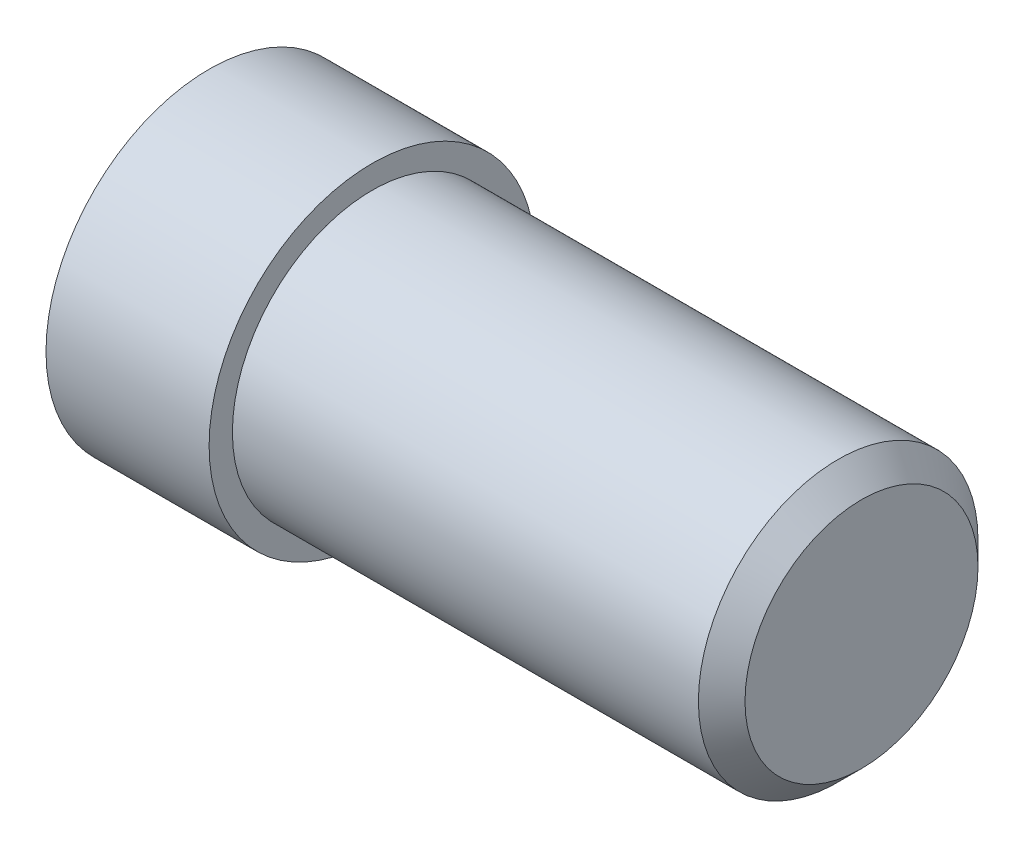
SolidWorks part; units mm, degrees
material "Plain Carbon Steel"
ref_plane "Front Plane" through (0, 0, 0) normal (0, 0, 1) x (1, 0, 0)
ref_plane "Top Plane" through (0, 0, 0) normal (0, 1, 0) x (1, 0, 0)
ref_plane "Right Plane" through (0, 0, 0) normal (1, 0, 0) x (0, 0, -1)
sketch "Bolt Profile Sketch" plane through (0, 0, 0) normal (0, 0, 1) x (1, 0, 0)
  line L0 (0, 0) -> (21, 0)
  line L1 (21, 0) -> (21, 6)
  line L2 (21, 6) -> (0, 6)
  line L3 (0, 6) -> (0, 7)
  line L4 (0, 7) -> (-7, 7)
  line L5 (-7, 7) -> (-7, 0)
  line L6 (-7, 0) -> (0, 0)
  dimension "D1" = 21
  dimension "D2" = 7
  dimension "D3" = 7
  dimension "D4" = 6
  dimension "D5" = 21
revolve "Bolt Body Revolve" add sketch "Bolt Profile Sketch" angle 360 about L0
chamfer "Shank Tip Chamfer 1x45°" distance 1 angle 45 1 edges at (21, 0, 6)
